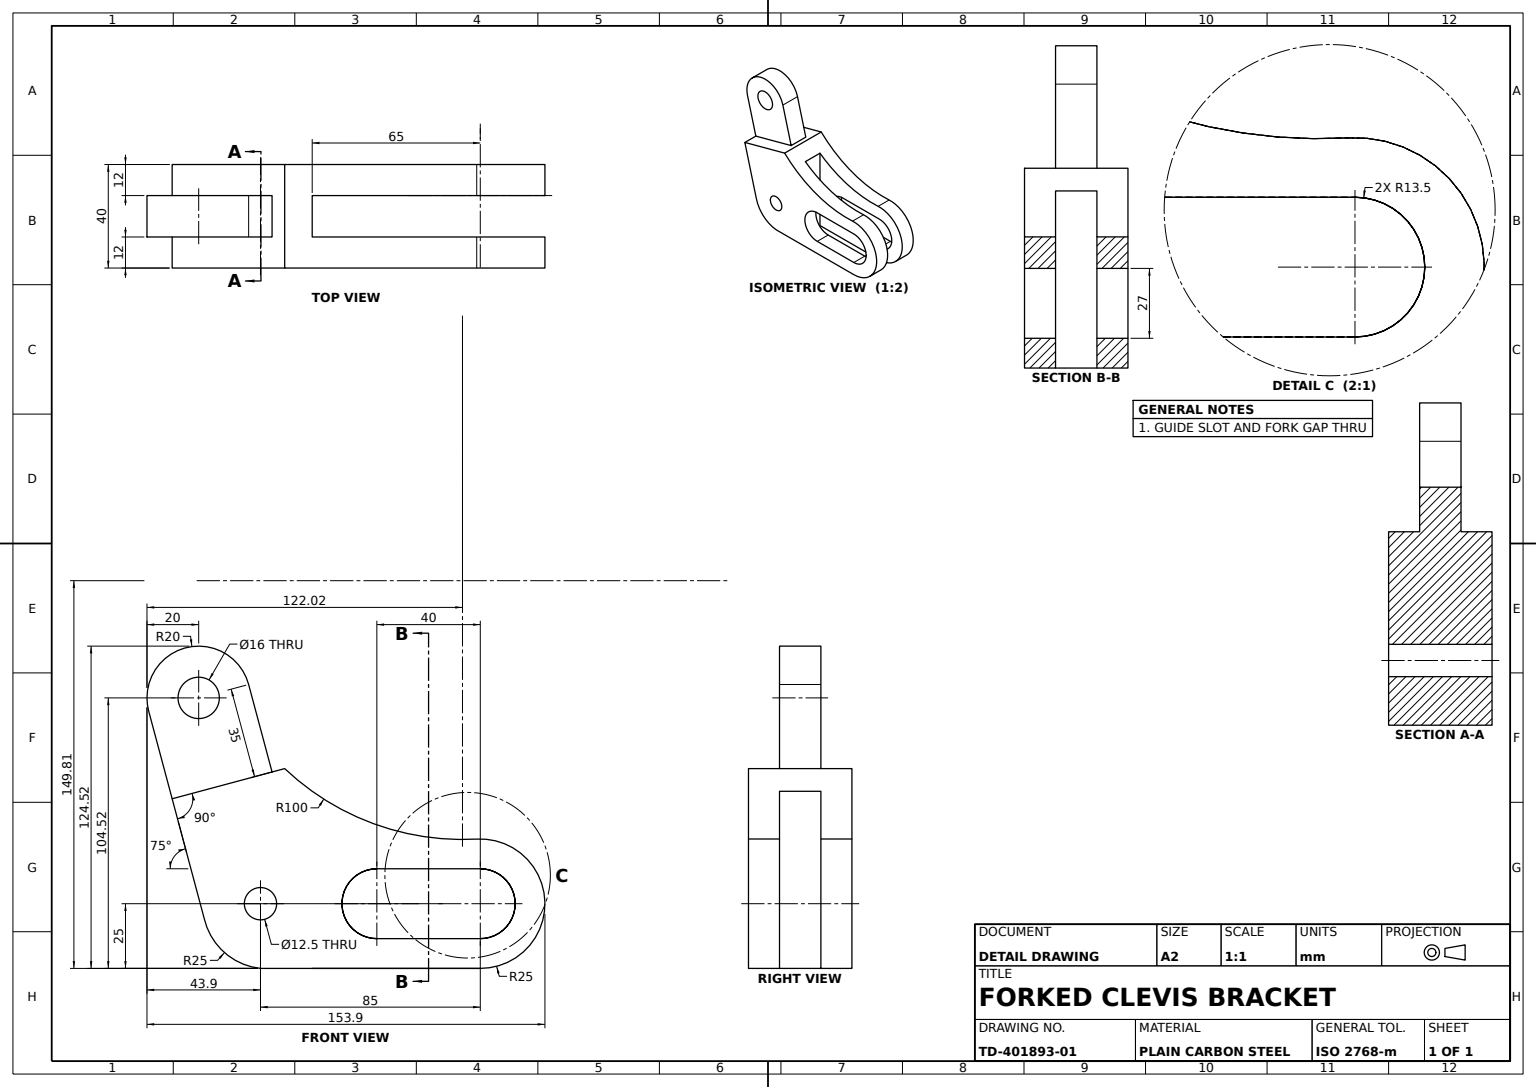
from build123d import *

# Parameters (mm, degrees)
BASE_PLATE_PROFILE_R = 6.25
BASE_PLATE_DEPTH     = 20
GUIDE_SLOT_DEPTH     = 137.100207792
FORK_GAP_16MM_DEPTH  = 8
PIVOT_LUG_DEPTH      = 8
PIVOT_HOLE_PROFILE_R = 8
PIVOT_HOLE_16_DEPTH  = 80


with BuildPart() as part:
    # Base Plate Profile → Base Plate (new, symmetric)
    with BuildSketch(Plane.XY):
        with BuildLine():
            Line((0, -25), (-85, -25))
            ThreePointArc((-85, -25), (-98.929277245, -18.882655563), (-106.733331092, -5.823428515))
            Line((-106.733331092, -5.823428515), (-119.156645256, 40.541011147))
            Line((-119.156645256, 40.541011147), (-75.640400658, 52.201153745))
            ThreePointArc((-75.640400658, 52.201153745), (-41.316083866, 30.926455065), (-1.376154737, 24.962095227))
            ThreePointArc((-1.376154737, 24.962095227), (24.99052201, 0.688338331), (0, -25))
        make_face()
        with Locations((-85, 0)):
            Circle(BASE_PLATE_PROFILE_R, mode=Mode.SUBTRACT)
    extrude(amount=BASE_PLATE_DEPTH, both=True)

    # Guide Slot Profile → Guide Slot (cut, through all)
    with BuildSketch(Plane.XY.offset(20)):
        with BuildLine():
            Line((-40, 13.5), (0, 13.5))
            ThreePointArc((0, 13.5), (13.5, 0), (0, -13.5))
            Line((0, -13.5), (-40, -13.5))
            ThreePointArc((-40, -13.5), (-53.5, 0), (-40, 13.5))
        make_face()
    extrude(amount=-GUIDE_SLOT_DEPTH, mode=Mode.SUBTRACT)

    # Fork Gap Profile → Fork Gap 16mm (cut, symmetric)
    with BuildSketch(Plane.XY):
        with BuildLine():
            Line((-65, 43.433848458), (-65, -25))
            Line((-65, -25), (0, -25))
            ThreePointArc((0, -25), (24.99052201, 0.688338331), (-1.376154737, 24.962095227))
            ThreePointArc((-1.376154737, 24.962095227), (-34.762230676, 28.775980481), (-65, 43.433848458))
        make_face()
    extrude(amount=FORK_GAP_16MM_DEPTH, both=True, mode=Mode.SUBTRACT)

    # Pivot Lug Profile → Pivot Lug (add, symmetric)
    with BuildSketch(Plane.XY):
        with BuildLine():
            Line((-119.156645256, 40.541011147), (-128.215311835, 74.348415067))
            ThreePointArc((-128.215311835, 74.348415067), (-114.073176211, 98.843312495), (-89.578278783, 84.701176871))
            Line((-89.578278783, 84.701176871), (-80.519612205, 50.893772951))
            Line((-80.519612205, 50.893772951), (-119.156645256, 40.541011147))
        make_face()
    extrude(amount=PIVOT_LUG_DEPTH, both=True)

    # Pivot Hole Profile → Pivot Hole Ø16 (cut, symmetric)
    with BuildSketch(Plane.XY.offset(8)):
        with Locations(Location((-108.896795309, 79.524795969, 0), (0, 0, 180))):
            Circle(PIVOT_HOLE_PROFILE_R)
    extrude(amount=PIVOT_HOLE_16_DEPTH, both=True, mode=Mode.SUBTRACT)


solid = part.part
